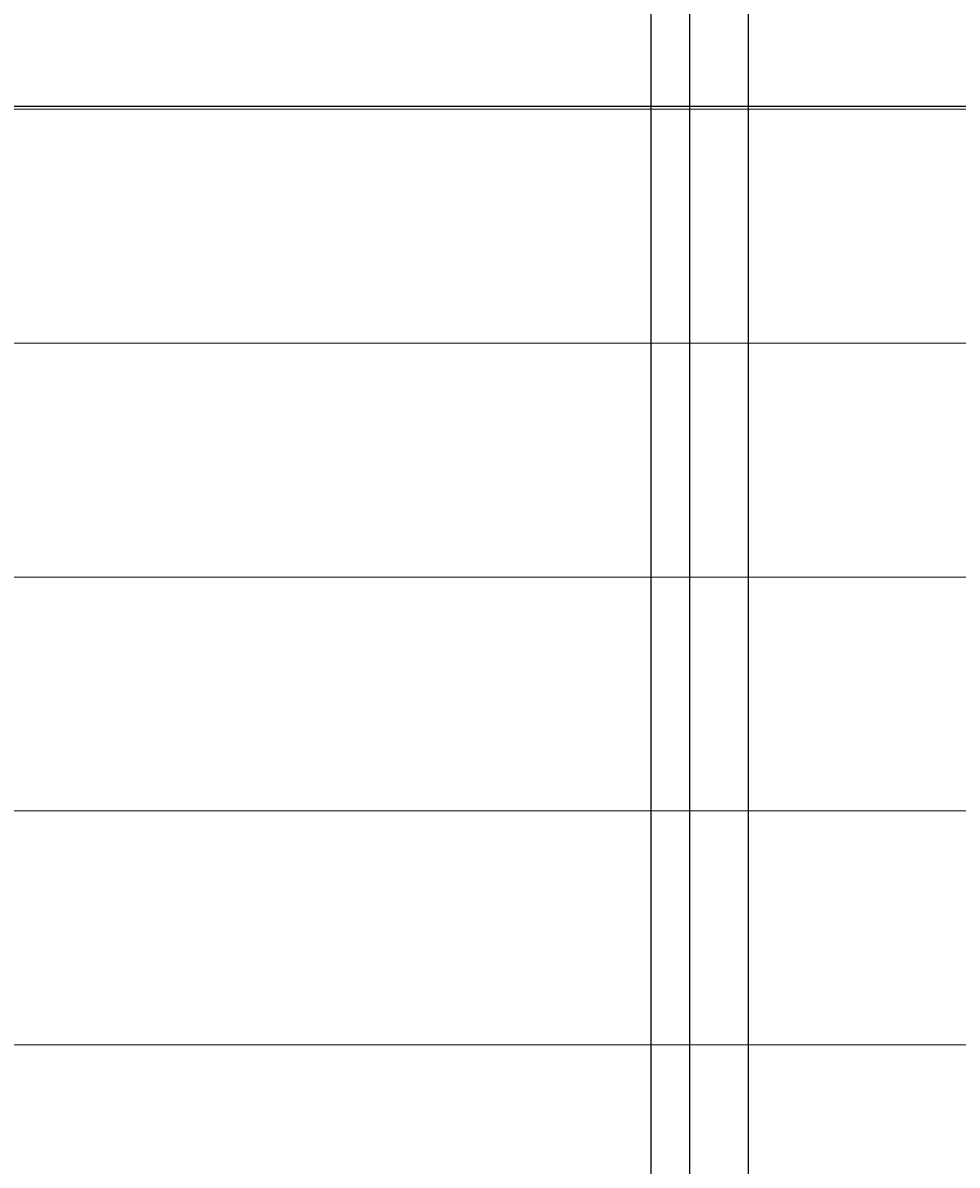
# Model space of a CAD drawing. Units: inches. Extents: x -6 to 289, y -8 to 323.
# Tile 19 of 107: x 150 to 174, y 21 to 50. Entities that reach past the tile are written whole.
import ezdxf

# ---------------------------------------------------------------- set-up
doc = ezdxf.new("R2010")
doc.units = ezdxf.units.IN
doc.header["$MEASUREMENT"] = 0
for name, color, linetype, lineweight in [('A-ANNO-DIMS', 2, 'Continuous', 18), ('A-DOOR', 3, 'Continuous', 25), ('A-ELEV-PATT', 8, 'Continuous', 13)]:
    doc.layers.add(name, color=color, linetype=linetype, lineweight=lineweight)
doc.styles.get("Standard").update_dxf_attribs({"font": 'arial.ttf'})
doc.dimstyles.get("Standard").update_dxf_attribs({"dimtxt": 0.18, "dimasz": 0.18, "dimexe": 0.18, "dimexo": 0.0625, "dimgap": 0.09, "dimtad": 0, "dimtih": 1, "dimtoh": 1, "dimdec": 4, "dimzin": 0, "dimdsep": 46, "dimtxsty": 'Standard', "dimcen": 0.09, "dimadec": 0, "dimazin": 0, "dimtfac": 1, "dimtdec": 4, "dimtofl": 0, "dimtmove": 0, "dimatfit": 3, "dimfxl": 1, "dimtolj": 1, "dimtzin": 0, "dimarcsym": 0})

# ---------------------------------------------------------------- blocks, each defined once
blk = doc.blocks.new('*D16')
at = {"layer": 'A-ANNO-DIMS', "color": 0, "lineweight": -2, "transparency": 16777216}
for p, q in [((9.943, 68.37), (9.943, -8.391)), ((272.973, 68.37), (272.973, -8.391)), ((10.123, -8.211), (140.993, -8.211)), ((272.793, -8.211), (141.923, -8.211))]:
    blk.add_line(p, q, dxfattribs=at)
at = {"layer": 'A-ANNO-DIMS', "color": 0, "transparency": 16777216}
for points in [[(10.123, -8.181), (10.123, -8.241), (9.943, -8.211)], [(272.793, -8.181), (272.793, -8.241), (272.973, -8.211)]]:
    blk.add_solid(points, dxfattribs=at)
at = {"layer": 'Defpoints', "color": 0, "transparency": 16777216}
for p in [(9.943, 68.432), (272.973, 68.432), (272.973, -8.211)]:
    blk.add_point(p, dxfattribs=at)
at = {"layer": 'A-ANNO-DIMS', "color": 0, "transparency": 16777216, "insert": (141.458, -8.211), "char_height": 0.18, "attachment_point": 5}
blk.add_mtext('\\A1;263.03', dxfattribs=at)
blk = doc.blocks.new('*D32')
at = {"layer": 'A-ANNO-DIMS', "color": 0, "lineweight": -2, "transparency": 16777216}
for p, q in [((147.883, 181.092), (147.883, -8.391)), ((166.383, 181.092), (166.383, -8.391)), ((148.063, -8.211), (156.817, -8.211)), ((166.203, -8.211), (157.449, -8.211))]:
    blk.add_line(p, q, dxfattribs=at)
at = {"layer": 'A-ANNO-DIMS', "color": 0, "transparency": 16777216}
for points in [[(148.063, -8.181), (148.063, -8.241), (147.883, -8.211)], [(166.203, -8.181), (166.203, -8.241), (166.383, -8.211)]]:
    blk.add_solid(points, dxfattribs=at)
at = {"layer": 'Defpoints', "color": 0, "transparency": 16777216}
for p in [(147.883, 181.154), (166.383, 181.154), (166.383, -8.211)]:
    blk.add_point(p, dxfattribs=at)
at = {"layer": 'A-ANNO-DIMS', "color": 0, "transparency": 16777216, "insert": (157.133, -8.211), "char_height": 0.18, "attachment_point": 5}
blk.add_mtext('\\A1;18.5', dxfattribs=at)
blk = doc.blocks.new('*D33')
at = {"layer": 'A-ANNO-DIMS', "color": 0, "lineweight": -2, "transparency": 16777216}
for p, q in [((166.383, 181.092), (166.383, -8.391)), ((167.383, 180.092), (167.383, -8.391)), ((166.563, -8.211), (166.76, -8.211)), ((167.203, -8.211), (167.007, -8.211))]:
    blk.add_line(p, q, dxfattribs=at)
at = {"layer": 'A-ANNO-DIMS', "color": 0, "transparency": 16777216}
for points in [[(166.563, -8.181), (166.563, -8.241), (166.383, -8.211)], [(167.203, -8.181), (167.203, -8.241), (167.383, -8.211)]]:
    blk.add_solid(points, dxfattribs=at)
at = {"layer": 'Defpoints', "color": 0, "transparency": 16777216}
for p in [(166.383, 181.154), (167.383, 180.154), (167.383, -8.211)]:
    blk.add_point(p, dxfattribs=at)
at = {"layer": 'A-ANNO-DIMS', "color": 0, "transparency": 16777216, "insert": (166.883, -8.211), "char_height": 0.18, "attachment_point": 5}
blk.add_mtext('\\A1;1', dxfattribs=at)
blk = doc.blocks.new('*D34')
at = {"layer": 'A-ANNO-DIMS', "color": 0, "lineweight": -2, "transparency": 16777216}
for p, q in [((167.383, 180.092), (167.383, -8.391)), ((168.883, 178.592), (168.883, -8.391)), ((167.563, -8.211), (167.887, -8.211)), ((168.703, -8.211), (168.38, -8.211))]:
    blk.add_line(p, q, dxfattribs=at)
at = {"layer": 'A-ANNO-DIMS', "color": 0, "transparency": 16777216}
for points in [[(167.563, -8.181), (167.563, -8.241), (167.383, -8.211)], [(168.703, -8.181), (168.703, -8.241), (168.883, -8.211)]]:
    blk.add_solid(points, dxfattribs=at)
at = {"layer": 'Defpoints', "color": 0, "transparency": 16777216}
for p in [(167.383, 180.154), (168.883, 178.654), (168.883, -8.211)]:
    blk.add_point(p, dxfattribs=at)
at = {"layer": 'A-ANNO-DIMS', "color": 0, "transparency": 16777216, "insert": (168.133, -8.211), "char_height": 0.18, "attachment_point": 5}
blk.add_mtext('\\A1;1.5', dxfattribs=at)

msp = doc.modelspace()

# ---------------------------------------------------------------- hatches: boundary and pattern name
at = {"layer": 'A-ELEV-PATT'}
h = msp.add_hatch(dxfattribs=at)
h.set_pattern_fill('_USER', color=256, scale=6, pattern_type=0)
h.set_pattern_definition([(0, (0, 0), (0, 6), [])])
h.paths.add_polyline_path([(184.1244, 48.0851), (124.008, 48.0851), (124.008, 10.2888), (184.1244, 10.2888)])
h.paths.add_polyline_path([(244.2408, 48.0851), (186.3604, 48.0851), (186.3604, 10.2888), (244.2408, 10.2888)])
h.paths.add_polyline_path([(208.2918, 114.2795), (190.7918, 114.2795), (190.7918, 71.2795), (208.2918, 71.2795)])
h.paths.add_polyline_path([(227.7918, 114.2795), (209.2918, 114.2795), (209.2918, 71.2795), (227.7918, 71.2795)])
h.paths.add_polyline_path([(211.2918, 224.3887), (190.7918, 224.3887), (190.7918, 162.3484), (211.2918, 162.3484)])
h.paths.add_polyline_path([(233.7918, 224.3887), (212.2918, 224.3887), (212.2918, 162.3484), (233.7918, 162.3484)])
h.paths.add_polyline_path([(166.3835, 224.154), (147.8835, 224.154), (147.8835, 181.154), (166.3835, 181.154)])
h.paths.add_polyline_path([(146.8835, 224.154), (129.3835, 224.154), (129.3835, 181.154), (146.8835, 181.154)])

# ---------------------------------------------------------------- linework, layer by layer
at = {"layer": 'A-DOOR'}
msp.add_lwpolyline([(124.008, 48.0851), (244.2408, 48.0851), (244.2408, 10.2888), (124.008, 10.2888)], close=True, dxfattribs=at)

# ---------------------------------------------------------------- dimensions: what is measured, and where the dimension line sits
at = {"layer": 'A-ANNO-DIMS'}
for base, p1, p2, override, picture, middle in [((166.3835, -8.2112), (147.8835, 181.154), (166.3835, 181.154), {"dimdec": 1, "dimlfac": 1, "dimrnd": 0, "dimzin": 0, "dimdsep": 46, "dimlunit": 2}, '*D32', (157.1335, -8.2112)), ((167.3835, -8.2112), (166.3835, 181.154), (167.3835, 180.154), {"dimdec": 0, "dimlfac": 1, "dimrnd": 0, "dimzin": 0, "dimdsep": 46, "dimlunit": 2}, '*D33', (166.8835, -8.2112)), ((168.8835, -8.2112), (167.3835, 180.154), (168.8835, 178.654), {"dimdec": 1, "dimlfac": 1, "dimrnd": 0, "dimzin": 0, "dimdsep": 46, "dimlunit": 2}, '*D34', (168.1335, -8.2112)), ((272.9733, -8.2112), (9.943, 68.4322), (272.9733, 68.4322), {"dimdec": 2, "dimlfac": 1, "dimrnd": 0, "dimzin": 0, "dimdsep": 46, "dimlunit": 2}, '*D16', (141.4581, -8.2112))]:
    dim = msp.add_linear_dim(base=base, p1=p1, p2=p2, dimstyle='Standard', override=override, dxfattribs=at)
    dim.commit()
    dim.dimension.update_dxf_attribs({"geometry": picture, "text_midpoint": middle})

doc.saveas('drawing.dxf')
